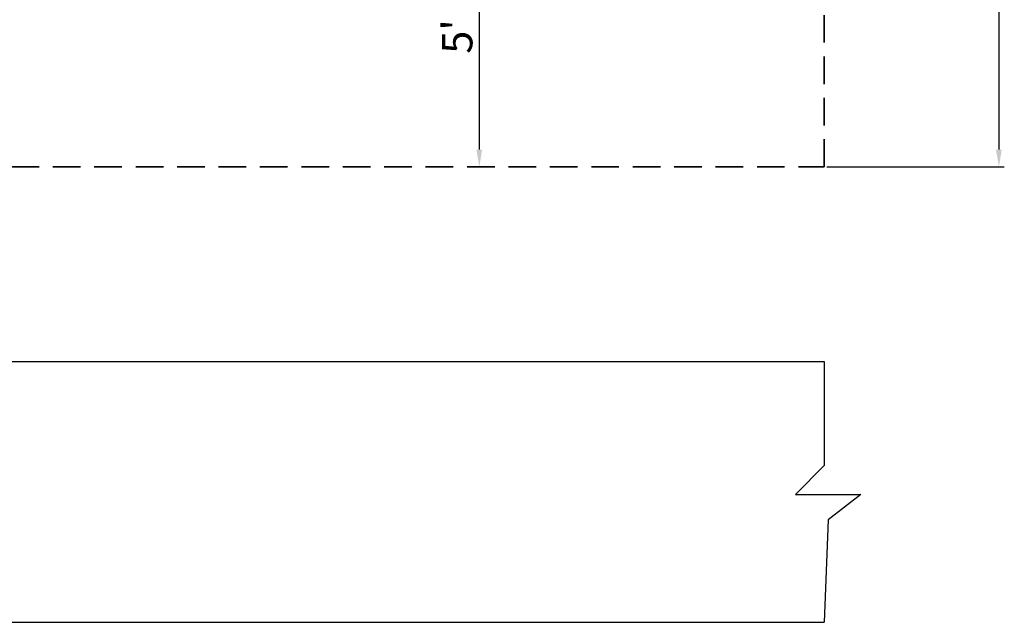
# Model space of a CAD drawing. Units: inches. Extents: x -7 to 1228, y -146 to 1091.
# Tile 35 of 88: x 1002 to 1228, y -105 to 34. Entities that reach past the tile are written whole.
import ezdxf

# ---------------------------------------------------------------- set-up
doc = ezdxf.new("R2010")
doc.units = ezdxf.units.IN
doc.linetypes.add('DASHED2', pattern=[9.525, 6.35, -3.175])
for name, color, linetype, lineweight in [('A-ANNO-DIMS', 2, 'Continuous', 18), ('C-PROP', 1, 'DASHED2', 35), ('C-ROAD', 7, 'Continuous', 25)]:
    doc.layers.add(name, color=color, linetype=linetype, lineweight=lineweight)
doc.styles.get("Standard").update_dxf_attribs({"font": 'arial.ttf'})
doc.dimstyles.new('ISO-25', dxfattribs={"dimtxt": 7, "dimasz": 4, "dimexe": 1.25, "dimexo": 0.625, "dimtad": 1, "dimdec": 1, "dimlunit": 3, "dimtxsty": 'Standard', "dimcen": 2.5, "dimadec": 0, "dimazin": 0, "dimtfac": 1, "dimtdec": 1, "dimtmove": 1, "dimatfit": 3, "dimfxl": 1, "dimarcsym": 0})

# ---------------------------------------------------------------- blocks, each defined once
blk = doc.blocks.new('*D12')
at = {"layer": 'A-ANNO-DIMS', "color": 0, "lineweight": -2, "transparency": 16777216}
for p, q in [((1187.62, 1061), (1228.45, 1061)), ((1227.2, 1057), (1227.2, 4)), ((1187.62, 0), (1228.45, 0))]:
    blk.add_line(p, q, dxfattribs=at)
at = {"layer": 'A-ANNO-DIMS', "color": 0, "transparency": 16777216}
for points in [[(1226.53, 1057), (1227.86, 1057), (1227.2, 1061)], [(1226.53, 4), (1227.86, 4), (1227.2, 0)]]:
    blk.add_solid(points, dxfattribs=at)
at = {"layer": 'Defpoints', "color": 0, "transparency": 16777216}
for p in [(1187, 1061), (1187, 0), (1227.2, 0)]:
    blk.add_point(p, dxfattribs=at)
at = {"layer": 'A-ANNO-DIMS', "color": 0, "transparency": 16777216, "insert": (1223, 530.5), "char_height": 7, "attachment_point": 5, "rotation": 90}
blk.add_mtext('88\'-5"', dxfattribs=at)
blk = doc.blocks.new('*D17')
at = {"layer": 'A-ANNO-DIMS', "color": 0, "lineweight": -2, "transparency": 16777216}
for p, q in [((1108.34, 60), (1108.96, 60)), ((1107.71, 56), (1107.71, 4)), ((1108.34, 0), (1108.96, 0))]:
    blk.add_line(p, q, dxfattribs=at)
at = {"layer": 'A-ANNO-DIMS', "color": 0, "transparency": 16777216}
for points in [[(1107.05, 56), (1108.38, 56), (1107.71, 60)], [(1107.05, 4), (1108.38, 4), (1107.71, 0)]]:
    blk.add_solid(points, dxfattribs=at)
at = {"layer": 'Defpoints', "color": 0, "transparency": 16777216}
for p in [(1107.71, 60), (1107.71, 0), (1107.71, 0)]:
    blk.add_point(p, dxfattribs=at)
at = {"layer": 'A-ANNO-DIMS', "color": 0, "transparency": 16777216, "insert": (1103.53, 30), "char_height": 7, "attachment_point": 5, "rotation": 90}
blk.add_mtext("5'", dxfattribs=at)

msp = doc.modelspace()

# ---------------------------------------------------------------- linework, layer by layer
at = {"layer": 'C-PROP'}
for p, q in [((1187, 0), (1187, 1061)), ((0, 0), (1187, 0))]:
    msp.add_line(p, q, dxfattribs=at)
at = {"layer": 'C-ROAD'}
for p, q in [((0, -44.69), (1187, -44.69)), ((1187, -44.69), (1187, -68.64)), ((1187, -68.64), (1180.43, -75.3)), ((1180.43, -75.3), (1195.46, -75.3)), ((1195.46, -75.3), (1187.95, -81.15)), ((1187.95, -81.15), (1187, -104.69)), ((0, -104.69), (1187, -104.69))]:
    msp.add_line(p, q, dxfattribs=at)

# ---------------------------------------------------------------- dimensions: what is measured, and where the dimension line sits
at = {"layer": 'A-ANNO-DIMS'}
for base, p1, p2, picture, middle in [((1227.2, 0), (1187, 1061), (1187, 0), '*D12', (1223, 530.5)), ((1107.71, 0), (1107.71, 60), (1107.71, 0), '*D17', (1103.53, 30))]:
    dim = msp.add_linear_dim(base=base, p1=p1, p2=p2, angle=90, dimstyle='ISO-25', override={"dimclrd": 0, "dimclre": 0, "dimclrt": 0}, dxfattribs=at)
    dim.commit()
    dim.dimension.update_dxf_attribs({"geometry": picture, "text_midpoint": middle})

doc.saveas('drawing.dxf')
